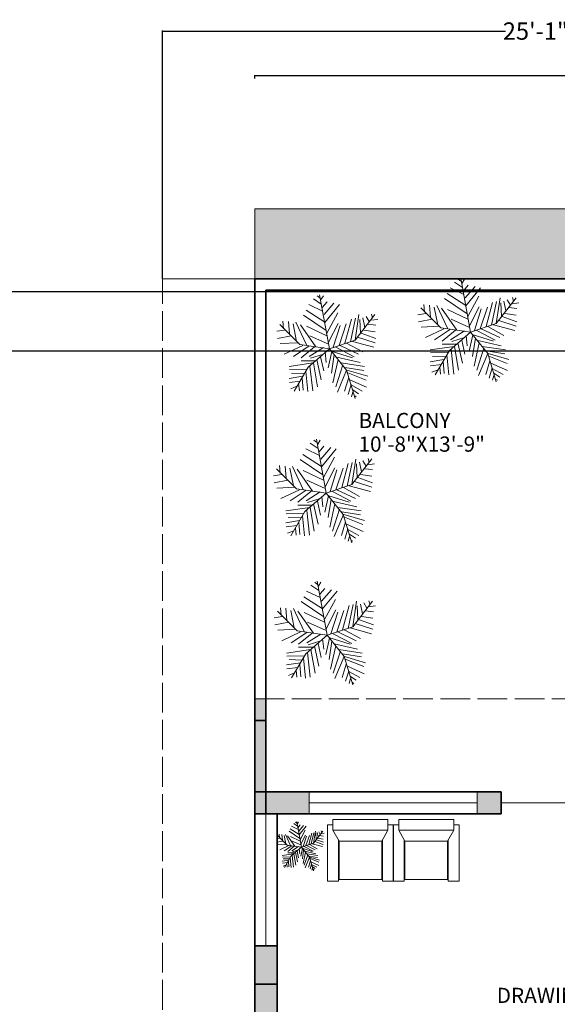
# Model space of a CAD drawing. Units: inches. Extents: x -17 to 892, y -721 to 172.
# Tile 8 of 11: x 438 to 655, y -231 to 166. Entities that reach past the tile are written whole.
import ezdxf

# ---------------------------------------------------------------- set-up
doc = ezdxf.new("R2010")
doc.units = ezdxf.units.IN
doc.header["$MEASUREMENT"] = 0
doc.linetypes.add('ACAD_ISO02W100', pattern=[15, 12, -3])
doc.layers.get('0').update_dxf_attribs({"color": 14})
for name, color, linetype, lineweight in [('A-ANNO-DIMS', 2, 'Continuous', 18), ('A-AREA-IDEN', 7, 'Continuous', 18), ('A-COLS', 252, 'Continuous', 35), ('A-FLOR-OVHD', 252, 'ACAD_ISO02W100', 18), ('A-WALL-PATT', 14, 'Continuous', 13), ('C-PROP', 8, 'ACAD_ISO02W100', 18), ('C-ROAD', 8, 'Continuous', 18), ('doors', 4, 'Continuous', 18), ('furniture', 252, 'Continuous', 18), ('lawn', 102, 'Continuous', 13), ('walls', 252, 'Continuous', 35), ('windows', 161, 'Continuous', 18)]:
    doc.layers.add(name, color=color, linetype=linetype, lineweight=lineweight)
doc.layers.add('A-COLS-PATT', color=254, linetype='Continuous', lineweight=13, true_color=0xd7ebd2)
doc.layers.add('C-ROAD-PATT', color=9, linetype='Continuous', lineweight=13, true_color=0xafd9aa)
doc.styles.get("Standard").update_dxf_attribs({"font": 'arial.ttf'})
doc.dimstyles.get("Standard").update_dxf_attribs({"dimtxt": 7, "dimasz": 0.18, "dimexe": 0.18, "dimexo": 0.0625, "dimgap": 0.09, "dimtad": 0, "dimtih": 1, "dimtoh": 1, "dimzin": 0, "dimdsep": 46, "dimlunit": 3, "dimtxsty": 'Standard', "dimcen": 0.09, "dimadec": 0, "dimazin": 0, "dimtfac": 1, "dimtofl": 0, "dimtmove": 0, "dimatfit": 3, "dimfxl": 1, "dimtolj": 1, "dimtzin": 0, "dimarcsym": 0})

# ---------------------------------------------------------------- blocks, each defined once
blk = doc.blocks.new('FABRIC SOFA 1S')
at = {"layer": 'furniture'}
for p, q in [((3, 18.12), (34, 18.12)), ((3, 15.12), (3, 18.12)), ((34, 12.12), (34, 18.12)), ((0, -15.12), (0, 15.12)), ((6, 15.12), (0, 15.12)), ((6, -15.12), (6, 15.12)), ((12, 11.75), (6, 15.12)), ((11.33, 12.12), (34, 12.12)), ((6, -15.12), (0, -15.12)), ((3, -18.12), (3, -15.12)), ((6, -15.12), (12, -11.75)), ((11.33, -12.12), (34, -12.12)), ((34, -12.12), (34, -18.12)), ((3, -18.12), (34, -18.12))]:
    blk.add_line(p, q, dxfattribs=at)
blk.add_lwpolyline([(12, -11.75), (12, 11.75), (33, 11.75), (33, -11.75)], close=True, dxfattribs=at)
blk = doc.blocks.new('*U14')
for p, q in [((-8.737, 47.138), (-17.069, 52.711)), ((-10.186, 53.64), (-13.084, 55.962)), ((0, 0), (-10.5, 57)), ((-9.099, 51.782), (-6.563, 55.962)), ((-7.288, 39.707), (-21.778, 46.673)), ((-7.65, 43.423), (-2.578, 49.46)), ((-5.839, 35.992), (4.667, 48.067)), ((-5.114, 27.632), (10.463, 46.673)), ((-3.665, 19.273), (-27.574, 35.527)), ((-5.114, 28.097), (-24.676, 40.636)), ((-2.941, 16.486), (8.652, 37.85)), ((16.259, 5.805), (23.142, 31.348)), ((22.055, 7.198), (27.489, 32.277)), ((27, 9), (48, 36)), ((27.127, 9.056), (31.112, 35.992)), ((35.096, 32.741), (37.27, 22.524)), ((38.719, 34.134), (41.979, 28.561)), ((44.153, 36.456), (45.239, 32.741)), ((-31.5, 4.5), (-52.5, 25.5)), ((-48.585, 21.131), (-49.309, 29.026)), ((-43.513, 28.561), (-42.427, 15.558)), ((-38.442, 26.239), (-34.819, 7.663)), ((-35.544, 28.097), (-24.314, 3.947)), ((-14.533, 2.09), (-30.834, 25.31)), ((-24.314, 23.917), (-2.941, 13.7)), ((-1.129, 6.734), (9.014, 26.704)), ((3.942, 1.625), (11.187, 24.381)), ((10.101, 3.483), (17.708, 26.239)), ((31.836, 30.883), (32.561, 16.486)), ((40.53, 25.775), (48.862, 24.846)), ((43.791, 29.954), (51.036, 30.883)), ((-47.498, 19.737), (-55.83, 18.344)), ((-40.615, 13.7), (-55.105, 10.913)), ((-20.691, 13.7), (-1.129, 4.876)), ((29.662, 12.307), (48.137, 6.269)), ((33.285, 16.486), (48.862, 10.913)), ((36.183, 19.737), (48.137, 17.88)), ((-33.37, 6.269), (-52.207, 5.34)), ((-28.299, 3.483), (-47.86, -5.805)), ((-21.416, 3.018), (-38.079, -8.128)), ((0, 0), (-31.5, 4.5)), ((-15.982, 2.09), (-30.11, -9.521)), ((0, 0), (-22.5, -19.5)), ((-6.563, 1.161), (-21.416, -8.128)), ((0, 0), (27, 9)), ((0, 0), (18, -22.5)), ((6.478, 1.625), (26.04, -8.592)), ((11.187, 3.483), (30.749, -5.805)), ((18.07, 5.805), (35.096, -3.483)), ((24.229, 7.663), (46.688, 1.625)), ((-6.563, -5.805), (-19.967, -9.985)), ((-9.461, -8.592), (-6.201, -23.453)), ((-4.752, -3.483), (-3.665, -14.629)), ((2.493, -3.019), (-1.491, -20.202)), ((1.769, -2.555), (24.229, -9.521)), ((5.029, -6.27), (2.131, -25.775)), ((7.565, -9.056), (32.198, -14.629)), ((-17.431, -15.094), (-42.789, -18.809)), ((-22.5, -19.5), (-37.5, -45)), ((-15.257, -12.772), (-30.11, -12.772)), ((-20.691, -18.345), (-17.793, -44.352)), ((-17.069, -15.094), (-12.721, -40.172)), ((-13.446, -11.378), (-8.737, -32.741)), ((9.014, -11.378), (3.58, -35.992)), ((14.085, -16.951), (6.478, -40.172)), ((12.274, -15.094), (36.907, -18.809)), ((16.259, -19.738), (36.183, -22.989)), ((-28.299, -29.026), (-42.789, -31.348)), ((-24.314, -21.596), (-42.427, -22.06)), ((-26.849, -26.24), (-40.253, -25.775)), ((-29.023, -30.884), (-27.936, -43.887)), ((-25.038, -23.918), (-22.865, -45.281)), ((18.07, -22.524), (8.289, -45.745)), ((20.244, -30.419), (15.897, -44.816)), ((18, -22.5), (27, -52.5)), ((18.433, -22.524), (40.53, -29.026)), ((19.157, -25.311), (38.719, -33.206)), ((-30.834, -34.135), (-42.427, -35.528)), ((-34.457, -39.708), (-40.978, -42.494)), ((-32.646, -36.921), (-31.921, -44.352)), ((22.78, -37.85), (19.519, -48.532)), ((21.331, -32.741), (39.081, -40.636)), ((22.78, -38.314), (34.372, -44.816)), ((24.591, -45.745), (23.142, -50.854)), ((24.591, -43.423), (30.749, -47.603)), ((26.764, -49.925), (28.213, -50.854))]:
    blk.add_line(p, q)
blk = doc.blocks.new('*D18')
at = {"layer": 'A-ANNO-DIMS', "color": 0, "lineweight": -2, "transparency": 16777216}
for p, q in [((532.58, 142.49), (532.58, 143.87)), ((532.76, 143.69), (658.49, 143.69)), ((796.4, 143.69), (670.67, 143.69)), ((796.58, 142.49), (796.58, 143.87))]:
    blk.add_line(p, q, dxfattribs=at)
at = {"layer": 'A-ANNO-DIMS', "color": 0, "lineweight": 100, "transparency": 16777216}
for points in [[(532.76, 143.72), (532.76, 143.66), (532.58, 143.69)], [(796.4, 143.72), (796.4, 143.66), (796.58, 143.69)]]:
    blk.add_solid(points, dxfattribs=at)
at = {"layer": 'Defpoints', "color": 0, "lineweight": 100, "transparency": 16777216}
for p in [(796.58, 143.69), (532.58, 142.43), (796.58, 142.43)]:
    blk.add_point(p, dxfattribs=at)
at = {"layer": 'A-ANNO-DIMS', "color": 0, "transparency": 16777216, "insert": (664.58, 143.69), "char_height": 7, "attachment_point": 5}
blk.add_mtext("\\A1;22'", dxfattribs=at)
blk = doc.blocks.new('WIN-68-INSET')
for p, q in [((0, 9), (0, 0)), ((0, 9), (0, 4.5)), ((67.89, 0), (67.89, 9)), ((0, 4.5), (67.89, 4.5))]:
    blk.add_line(p, q)
blk = doc.blocks.new('WIN-53-INSET')
for p, q in [((0, 53.21), (9, 53.21)), ((0, 53.21), (4.5, 53.21)), ((4.5, 53.21), (4.5, 0)), ((9, 0), (0, 0))]:
    blk.add_line(p, q)
blk = doc.blocks.new('*D58')
at = {"layer": 'A-ANNO-DIMS', "color": 0, "lineweight": -2, "transparency": 16777216}
for p, q in [((495.38, 61.67), (495.38, 161.84)), ((495.56, 161.66), (633.81, 161.66)), ((796.4, 161.66), (658.15, 161.66)), ((796.58, 89.96), (796.58, 161.84))]:
    blk.add_line(p, q, dxfattribs=at)
at = {"layer": 'A-ANNO-DIMS', "color": 0, "lineweight": 100, "transparency": 16777216}
for points in [[(495.56, 161.69), (495.56, 161.63), (495.38, 161.66)], [(796.4, 161.69), (796.4, 161.63), (796.58, 161.66)]]:
    blk.add_solid(points, dxfattribs=at)
at = {"layer": 'Defpoints', "color": 0, "lineweight": 100, "transparency": 16777216}
for p in [(796.58, 161.66), (796.58, 89.9), (495.38, 61.61)]:
    blk.add_point(p, dxfattribs=at)
at = {"layer": 'A-ANNO-DIMS', "color": 0, "transparency": 16777216, "insert": (645.98, 161.66), "char_height": 7, "attachment_point": 5}
blk.add_mtext('\\A1;25\'-1"', dxfattribs=at)
blk = doc.blocks.new('*D68')
at = {"layer": 'A-ANNO-DIMS', "color": 0, "lineweight": -2, "transparency": 16777216}
for p, q in [((738.65, 56.46), (1.11, 56.46)), ((1.29, 56.28), (1.29, 48.13)), ((1.29, 32.64), (1.29, 40.8)), ((737.65, 32.46), (1.11, 32.46))]:
    blk.add_line(p, q, dxfattribs=at)
at = {"layer": 'A-ANNO-DIMS', "color": 0, "lineweight": 100, "transparency": 16777216}
for points in [[(1.26, 56.28), (1.32, 56.28), (1.29, 56.46)], [(1.26, 32.64), (1.32, 32.64), (1.29, 32.46)]]:
    blk.add_solid(points, dxfattribs=at)
at = {"layer": 'Defpoints', "color": 0, "lineweight": 100, "transparency": 16777216}
for p in [(738.71, 56.46), (1.29, 32.46), (737.71, 32.46)]:
    blk.add_point(p, dxfattribs=at)
at = {"layer": 'A-ANNO-DIMS', "color": 0, "transparency": 16777216, "insert": (1.29, 44.46), "char_height": 7, "attachment_point": 5}
blk.add_mtext('\\A1;2\'-0"', dxfattribs=at)

msp = doc.modelspace()

# ---------------------------------------------------------------- hatches: boundary and pattern name
at = {"layer": 'A-COLS-PATT'}
h = msp.add_hatch(color=256, dxfattribs=at)
h.dxf.hatch_style = 1
h.paths.add_polyline_path([(796.576, 61.611), (787.576, 61.611), (787.576, 43.692), (796.576, 43.692)])
h.paths.add_polyline_path([(796.576, -140.181), (787.576, -140.181), (787.576, -157.529), (796.576, -157.529)])
h.paths.add_polyline_path([(674.076, -107.889), (665.076, -107.889), (665.076, -116.615), (674.076, -116.615)])
h.paths.add_polyline_path([(537.076, -107.889), (532.576, -107.889), (532.576, -116.615), (537.076, -116.615)])
h.paths.add_polyline_path([(541.576, -207.597), (532.576, -207.597), (532.576, -223.04), (541.576, -223.04)])
h.paths.add_polyline_path([(541.576, -335.389), (532.576, -335.389), (532.576, -350.421), (541.576, -350.421)])
h.paths.add_polyline_path([(541.576, -412.049), (532.576, -412.049), (532.576, -420.971), (541.576, -420.971)])
h.paths.add_polyline_path([(674.076, -410.999), (665.076, -410.999), (665.076, -421.003), (674.076, -421.003)])
h.paths.add_polyline_path([(674.076, -329.432), (665.076, -329.432), (665.076, -335.389), (665.076, -343.822), (674.076, -343.822), (674.076, -335.389)])
h.paths.add_polyline_path([(667.076, -610.134), (659.076, -610.134), (659.076, -618.889), (659.101, -623.389), (667.076, -623.389)])
h.paths.add_polyline_path([(796.576, -610.134), (787.576, -610.134), (787.576, -614.389), (787.576, -623.342), (796.576, -623.342)])
h.paths.add_polyline_path([(796.576, -324.682), (787.576, -324.682), (787.576, -353.487), (796.576, -353.487)])
at = {"layer": 'A-WALL-PATT'}
h = msp.add_hatch(color=256, dxfattribs=at)
h.dxf.hatch_style = 1
h.paths.add_polyline_path([(669.576, 4.611), (787.576, 4.611), (787.576, 9.111), (669.576, 9.111), (669.576, 53.097), (665.076, 53.097), (665.076, -107.889), (669.576, -107.889)])
h.paths.add_polyline_path([(674.076, -116.615), (665.076, -116.615), (665.076, -154.389), (674.076, -154.389)])
h.paths.add_polyline_path([(787.576, -145.389), (713.344, -145.389), (713.344, -154.389), (787.576, -154.389)])
h.paths.add_polyline_path([(632.137, -145.389), (622.476, -145.389), (622.476, -154.389), (632.137, -154.389)])
h.paths.add_polyline_path([(554.583, -145.389), (537.076, -145.389), (537.076, -154.389), (554.583, -154.389)])
h.paths.add_polyline_path([(537.076, -145.389), (532.576, -145.389), (532.576, -154.389), (537.076, -154.389)])
h.paths.add_polyline_path([(537.076, -116.615), (532.576, -116.615), (532.576, -145.389), (537.076, -145.389)])
h.paths.add_polyline_path([(796.576, 43.692), (787.576, 43.692), (787.576, -140.181), (796.576, -140.181)])
h.paths.add_polyline_path([(541.576, -223.04), (532.576, -223.04), (532.576, -282.182), (537.076, -282.182), (541.576, -282.182)])
h.paths.add_polyline_path([(796.576, -157.529), (787.576, -157.529), (787.576, -324.682), (796.576, -324.682)])
h.paths.add_polyline_path([(554.583, -335.389), (541.576, -335.389), (541.576, -344.389), (554.583, -344.389)])
h.paths.add_polyline_path([(635.731, -335.389), (622.476, -335.389), (622.476, -344.389), (635.731, -344.389)])
h.paths.add_polyline_path([(541.576, -350.421), (532.576, -350.421), (532.576, -412.049), (541.576, -412.049)])
h.paths.add_polyline_path([(674.076, -343.822), (665.076, -343.822), (665.076, -410.999), (674.076, -410.999)])
h.paths.add_polyline_path([(667.076, -421.003), (665.076, -421.003), (659.076, -421.002), (659.076, -610.134), (667.076, -610.134)])
h.paths.add_polyline_path([(796.576, -353.487), (787.576, -353.487), (787.576, -610.134), (796.576, -610.134)])
h.paths.add_polyline_path([(787.576, -335.389), (775.362, -335.389), (775.362, -344.389), (787.576, -344.389)])
h.paths.add_polyline_path([(707.469, -335.389), (703.501, -335.389), (703.501, -344.389), (707.469, -344.389)])
h.paths.add_polyline_path([(695.494, 61.611), (676.541, 61.611), (676.541, 57.111), (695.494, 57.111)])
h.paths.add_polyline_path([(729.183, 61.611), (724.076, 61.611), (711.12, 61.611), (711.12, 57.111), (729.183, 57.111)])
h.paths.add_polyline_path([(787.576, 61.611), (735.904, 61.611), (735.904, 57.111), (787.576, 57.111)])
at = {"layer": 'C-ROAD-PATT'}
h = msp.add_hatch(dxfattribs=at)
h.set_pattern_fill('BRICK', color=256)
h.set_pattern_definition([(0, (449.49168, 0), (0, 0.25), []), (90, (449.4917, 0), (-0.5, 0), [0.25, -0.25]), (90, (449.7417, 0), (-0.5, 0), [-0.25, 0.25])])
h.paths.add_polyline_path([(796.576, 89.902), (532.576, 89.902), (532.576, 61.611), (796.576, 61.611)])

# ---------------------------------------------------------------- linework, layer by layer
at = {"layer": 'A-COLS'}
for p, q in [((532.576, -116.615), (537.076, -116.615)), ((532.576, -207.597), (541.576, -207.597)), ((532.576, -223.04), (541.576, -223.04))]:
    msp.add_line(p, q, dxfattribs=at)
at = {"layer": 'A-FLOR-OVHD'}
msp.add_line((532.576, -107.889), (674.076, -107.889), dxfattribs=at)
at = {"layer": 'C-PROP'}
msp.add_line((495.384, -623.389), (495.384, 61.611), dxfattribs=at)
at = {"layer": 'C-ROAD'}
for p, q in [((532.576, 61.611), (532.576, 89.902)), ((532.576, 89.902), (796.576, 89.902)), ((495.384, 61.611), (532.576, 61.611))]:
    msp.add_line(p, q, dxfattribs=at)
at = {"layer": 'doors'}
msp.add_line((632.137, -149.889), (665.076, -149.889), dxfattribs=at)
at = {"layer": 'walls'}
for p, q in [((532.576, 61.611), (796.576, 61.611)), ((532.576, -623.389), (532.576, 61.611)), ((537.076, 57.111), (787.576, 57.111)), ((537.076, -154.389), (537.076, 57.111)), ((532.576, -145.389), (632.137, -145.389)), ((632.137, -145.389), (632.137, -154.389)), ((532.576, -154.389), (632.137, -154.389)), ((541.576, -420.971), (541.576, -154.389))]:
    msp.add_line(p, q, dxfattribs=at)

# ---------------------------------------------------------------- block references
at = {"layer": 'furniture', "xscale": -0.7339463821036302, "yscale": 0.7339463821036302, "zscale": 0.7339463821036302}
for p, rotation in [((575.261, -156.577), 89.99999999999912), ((601.866, -156.577), 90)]:
    msp.add_blockref('FABRIC SOFA 1S', p, dxfattribs=dict(at, rotation=rotation))
at = {"layer": 'lawn'}
for p, xscale, yscale, zscale in [((619.788, 40.153), 0.3823150569682844, 0.3823150569682844, 0.3823150569682844), ((562.8, 33.439), 0.3823150569682844, 0.3823150569682844, 0.3823150569682844), ((561.484, -24.85), 0.3823150569682844, 0.3823150569682844, 0.3823150569682844), ((561.829, -82.226), 0.3823150569682844, 0.3823150569682844, 0.3823150569682844), ((551.432, -167.796), 0.1813548619598531, 0.1813548619598531, 0.1813548619598531)]:
    msp.add_blockref('*U14', p, dxfattribs=dict(at, xscale=xscale, yscale=yscale, zscale=zscale))
at = {"layer": 'windows'}
for name, p in [('WIN-68-INSET', (554.583, -154.389)), ('WIN-53-INSET', (532.576, -207.597))]:
    msp.add_blockref(name, p, dxfattribs=at)

# ---------------------------------------------------------------- texts
at = {"layer": 'A-AREA-IDEN'}
for s, p in [('BALCONY', (574.506, 1.393)), ('10\'-8"X13\'-9"', (574.506, -8.142)), ('DRAWING ROOM', (630.34, -230.702))]:
    msp.add_text(s, height=6.1361, dxfattribs=at).set_placement(p)

# ---------------------------------------------------------------- dimensions: what is measured, and where the dimension line sits
at = {"layer": 'A-ANNO-DIMS'}
for base, p1, p2, override, picture, middle in [((796.576, 161.663), (495.384, 61.611), (796.576, 89.902), {"dimdec": 1, "dimlfac": 1, "dimrnd": 0, "dimzin": 1, "dimdsep": 46, "dimlunit": 4, "dimfrac": 2}, '*D58', (645.98, 161.663)), ((796.576, 143.692), (532.576, 142.427), (796.576, 142.427), {"dimclrd": 0, "dimclre": 0, "dimclrt": 0}, '*D18', (664.576, 143.692))]:
    dim = msp.add_linear_dim(base=base, p1=p1, p2=p2, dimstyle='Standard', override=override, dxfattribs=at)
    dim.commit()
    dim.dimension.update_dxf_attribs({"geometry": picture, "text_midpoint": middle})
dim = msp.add_linear_dim(base=(1.292, 32.461), p1=(738.709, 56.461), p2=(737.709, 32.461), angle=90, dimstyle='Standard', override={"dimdec": 1, "dimlfac": 1, "dimrnd": 0, "dimzin": 1, "dimdsep": 46, "dimlunit": 4, "dimfrac": 2}, dxfattribs=at)
dim.commit()
dim.dimension.update_dxf_attribs({"geometry": '*D68', "text_midpoint": (1.292, 44.461)})

doc.saveas('drawing.dxf')
